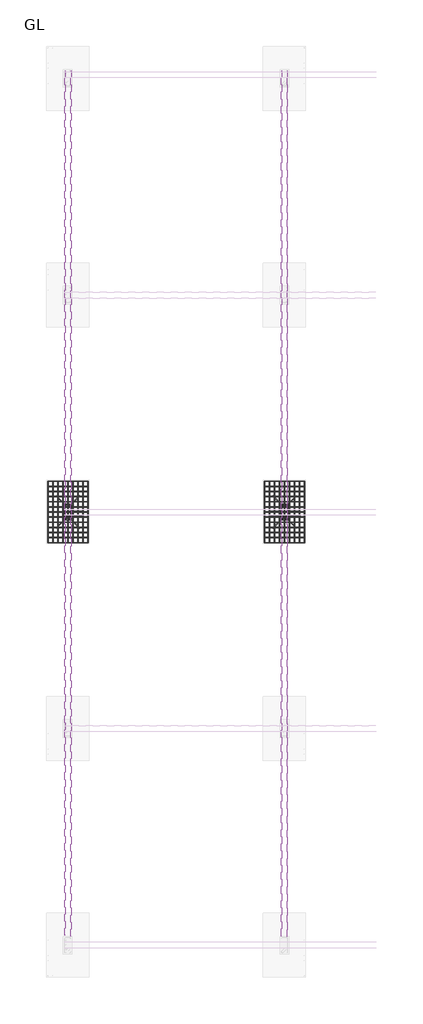
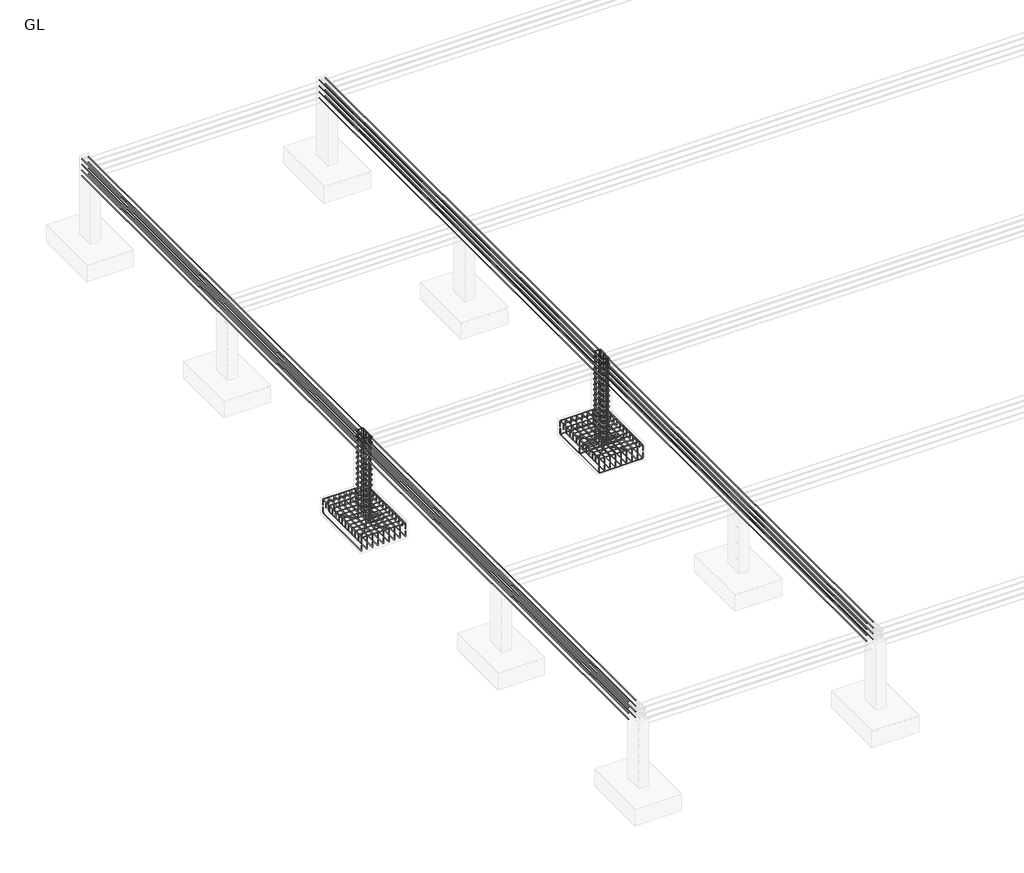
# One storey, part 5 of 16: 24 reinforcing bars.
"""IFC4 building model written with IfcOpenShell, lengths in millimetres."""

from ifc_helpers import new_model, si_unit, point, frame, origin, place, context, project, spatial, polyline, circle_curve, trimmed, segment, composite_curve, source, transform, mapped, element, save
from ifc_brep_helpers import swept_disk

model = new_model("IFC4")

# Units and contexts
model_context = context("Model", 3, world=origin())
ifc_project = project(units=[si_unit("LENGTHUNIT", "METRE", prefix="MILLI")], contexts=[model_context])

# Site, building, storey
site = spatial("IfcSite", under=ifc_project)
building = spatial("IfcBuilding", under=site)
storey = spatial("IfcBuildingStorey", under=building, Name="GL", Elevation=-1829.0)

# Reinforcing bars
placement = place(None, origin())
reinforcing_bar_shape = source(origin(), model_context, "Body", "SolidModel", [
    swept_disk(composite_curve([segment(polyline([(-23370.9544379, -7223.1167521, -2022.436678), (-23370.9544379, -7223.1167521, -1898.436678)]), True, "CONTINUOUS"), segment(trimmed(circle_curve(frame((-23340.9544379, -7223.1167521, -1898.436678), z_axis=(0.0, 1.0, 0.0), x_axis=(-30.0, 0.0, 0.0)), 30.0), [point((-23370.9544379, -7223.1167521, -1898.436678))], [point((-23340.9544379, -7223.1167521, -1868.436678))], True, "CARTESIAN"), True, "CONTINUOUS"), segment(polyline([(-23340.9544379, -7223.1167521, -1868.436678), (-22272.9544379, -7223.1167521, -1868.436678)]), True, "CONTINUOUS"), segment(trimmed(circle_curve(frame((-22272.9544379, -7223.1167521, -1898.436678), z_axis=(0.0, 1.0, 0.0), x_axis=(0.0, 0.0, 30.0)), 30.0), [point((-22272.9544379, -7223.1167521, -1868.436678))], [point((-22242.9544379, -7223.1167521, -1898.436678))], True, "CARTESIAN"), True, "CONTINUOUS"), segment(polyline([(-22242.9544379, -7223.1167521, -1898.436678), (-22242.9544379, -7223.1167521, -2022.436678)]), True, "CONTINUOUS")], self_intersect=False), 6.0),
])
element("IfcReinforcingBar", 1, at=placement, inside=storey, context=model_context, shape_type="MappedRepresentation", body=[
    mapped(reinforcing_bar_shape, transform((0.0, 0.0, 0.0), x_axis=(1.0, 0.0, 0.0), y_axis=(0.0, 1.0, 0.0), z_axis=(0.0, 0.0, 1.0))),
    mapped(reinforcing_bar_shape, transform((0.0, -144.0, 0.0), x_axis=(1.0, 0.0, 0.0), y_axis=(0.0, 1.0, 0.0), z_axis=(0.0, 0.0, 1.0))),
    mapped(reinforcing_bar_shape, transform((0.0, -288.0, 0.0), x_axis=(1.0, 0.0, 0.0), y_axis=(0.0, 1.0, 0.0), z_axis=(0.0, 0.0, 1.0))),
    mapped(reinforcing_bar_shape, transform((0.0, -432.0, 0.0), x_axis=(1.0, 0.0, 0.0), y_axis=(0.0, 1.0, 0.0), z_axis=(0.0, 0.0, 1.0))),
    mapped(reinforcing_bar_shape, transform((0.0, -576.0, 0.0), x_axis=(1.0, 0.0, 0.0), y_axis=(0.0, 1.0, 0.0), z_axis=(0.0, 0.0, 1.0))),
    mapped(reinforcing_bar_shape, transform((0.0, -720.0, 0.0), x_axis=(1.0, 0.0, 0.0), y_axis=(0.0, 1.0, 0.0), z_axis=(0.0, 0.0, 1.0))),
    mapped(reinforcing_bar_shape, transform((0.0, -864.0, 0.0), x_axis=(1.0, 0.0, 0.0), y_axis=(0.0, 1.0, 0.0), z_axis=(0.0, 0.0, 1.0))),
    mapped(reinforcing_bar_shape, transform((0.0, -1008.0, 0.0), x_axis=(1.0, 0.0, 0.0), y_axis=(0.0, 1.0, 0.0), z_axis=(0.0, 0.0, 1.0))),
    mapped(reinforcing_bar_shape, transform((0.0, -1152.0, 0.0), x_axis=(1.0, 0.0, 0.0), y_axis=(0.0, 1.0, 0.0), z_axis=(0.0, 0.0, 1.0))),
    mapped(reinforcing_bar_shape, transform((0.0, -1296.0, 0.0), x_axis=(1.0, 0.0, 0.0), y_axis=(0.0, 1.0, 0.0), z_axis=(0.0, 0.0, 1.0))),
    mapped(reinforcing_bar_shape, transform((0.0, -1440.0, 0.0), x_axis=(1.0, 0.0, 0.0), y_axis=(0.0, 1.0, 0.0), z_axis=(0.0, 0.0, 1.0))),
    mapped(reinforcing_bar_shape, transform((0.0, -1584.0, 0.0), x_axis=(1.0, 0.0, 0.0), y_axis=(0.0, 1.0, 0.0), z_axis=(0.0, 0.0, 1.0))),
    mapped(reinforcing_bar_shape, transform((0.0, -1728.0, 0.0), x_axis=(1.0, 0.0, 0.0), y_axis=(0.0, 1.0, 0.0), z_axis=(0.0, 0.0, 1.0))),
])
reinforcing_bar_2_shape = source(origin(), model_context, "Body", "SolidModel", [
    swept_disk(composite_curve([segment(polyline([(-23370.9544379, -8951.1167521, -2027.5081232), (-23370.9544379, -8951.1167521, -1903.5081232)]), True, "CONTINUOUS"), segment(trimmed(circle_curve(frame((-23370.9544379, -8921.1167521, -1903.5081232), z_axis=(-1.0, 0.0, 0.0), x_axis=(0.0, -30.0, 0.0)), 30.0), [point((-23370.9544379, -8951.1167521, -1903.5081232))], [point((-23370.9544379, -8921.1167521, -1873.5081232))], True, "CARTESIAN"), True, "CONTINUOUS"), segment(polyline([(-23370.9544379, -8921.1167521, -1873.5081232), (-23370.9544379, -7253.1167521, -1873.5081232)]), True, "CONTINUOUS"), segment(trimmed(circle_curve(frame((-23370.9544379, -7253.1167521, -1903.5081232), z_axis=(-1.0, 0.0, 0.0), x_axis=(0.0, 0.0, 30.0)), 30.0), [point((-23370.9544379, -7253.1167521, -1873.5081232))], [point((-23370.9544379, -7223.1167521, -1903.5081232))], True, "CARTESIAN"), True, "CONTINUOUS"), segment(polyline([(-23370.9544379, -7223.1167521, -1903.5081232), (-23370.9544379, -7223.1167521, -2027.5081232)]), True, "CONTINUOUS")], self_intersect=False), 6.0),
])
element("IfcReinforcingBar", 2, at=placement, inside=storey, context=model_context, shape_type="MappedRepresentation", body=[
    mapped(reinforcing_bar_2_shape, transform((0.0, 0.0, 0.0), x_axis=(1.0, 0.0, 0.0), y_axis=(0.0, 1.0, 0.0), z_axis=(0.0, 0.0, 1.0))),
    mapped(reinforcing_bar_2_shape, transform((141.0, 0.0, 0.0), x_axis=(1.0, 0.0, 0.0), y_axis=(0.0, 1.0, 0.0), z_axis=(0.0, 0.0, 1.0))),
    mapped(reinforcing_bar_2_shape, transform((282.0, 0.0, 0.0), x_axis=(1.0, 0.0, 0.0), y_axis=(0.0, 1.0, 0.0), z_axis=(0.0, 0.0, 1.0))),
    mapped(reinforcing_bar_2_shape, transform((423.0, 0.0, 0.0), x_axis=(1.0, 0.0, 0.0), y_axis=(0.0, 1.0, 0.0), z_axis=(0.0, 0.0, 1.0))),
    mapped(reinforcing_bar_2_shape, transform((564.0, 0.0, 0.0), x_axis=(1.0, 0.0, 0.0), y_axis=(0.0, 1.0, 0.0), z_axis=(0.0, 0.0, 1.0))),
    mapped(reinforcing_bar_2_shape, transform((705.0, 0.0, 0.0), x_axis=(1.0, 0.0, 0.0), y_axis=(0.0, 1.0, 0.0), z_axis=(0.0, 0.0, 1.0))),
    mapped(reinforcing_bar_2_shape, transform((846.0, 0.0, 0.0), x_axis=(1.0, 0.0, 0.0), y_axis=(0.0, 1.0, 0.0), z_axis=(0.0, 0.0, 1.0))),
    mapped(reinforcing_bar_2_shape, transform((987.0, 0.0, 0.0), x_axis=(1.0, 0.0, 0.0), y_axis=(0.0, 1.0, 0.0), z_axis=(0.0, 0.0, 1.0))),
    mapped(reinforcing_bar_2_shape, transform((1128.0, 0.0, 0.0), x_axis=(1.0, 0.0, 0.0), y_axis=(0.0, 1.0, 0.0), z_axis=(0.0, 0.0, 1.0))),
])
reinforcing_bar_3_shape = source(origin(), model_context, "Body", "SolidModel", [
    swept_disk(composite_curve([segment(polyline([(-22242.9544379, -8951.1167521, -2080.6239909), (-22242.9544379, -8951.1167521, -2204.6239909)]), True, "CONTINUOUS"), segment(trimmed(circle_curve(frame((-22242.9544379, -8921.1167521, -2204.6239909), z_axis=(1.0, 0.0, 0.0), x_axis=(0.0, -30.0, 0.0)), 30.0), [point((-22242.9544379, -8951.1167521, -2204.6239909))], [point((-22242.9544379, -8921.1167521, -2234.6239909))], True, "CARTESIAN"), True, "CONTINUOUS"), segment(polyline([(-22242.9544379, -8921.1167521, -2234.6239909), (-22242.9544379, -7266.1421892, -2234.6239909)]), True, "CONTINUOUS"), segment(trimmed(circle_curve(frame((-22242.9544379, -7266.1421892, -2204.6239909), z_axis=(1.0, 0.0, 0.0), x_axis=(0.0, 0.0, -30.0)), 30.0), [point((-22242.9544379, -7266.1421892, -2234.6239909))], [point((-22242.9544379, -7236.1421892, -2204.6239909))], True, "CARTESIAN"), True, "CONTINUOUS"), segment(polyline([(-22242.9544379, -7236.1421892, -2204.6239909), (-22242.9544379, -7236.1421892, -2080.6239909)]), True, "CONTINUOUS")], self_intersect=False), 6.0),
])
element("IfcReinforcingBar", 3, at=placement, inside=storey, context=model_context, shape_type="MappedRepresentation", body=[
    mapped(reinforcing_bar_3_shape, transform((0.0, 0.0, 0.0), x_axis=(1.0, 0.0, 0.0), y_axis=(0.0, 1.0, 0.0), z_axis=(0.0, 0.0, 1.0))),
    mapped(reinforcing_bar_3_shape, transform((-141.0, 0.0, 0.0), x_axis=(1.0, 0.0, 0.0), y_axis=(0.0, 1.0, 0.0), z_axis=(0.0, 0.0, 1.0))),
    mapped(reinforcing_bar_3_shape, transform((-282.0, 0.0, 0.0), x_axis=(1.0, 0.0, 0.0), y_axis=(0.0, 1.0, 0.0), z_axis=(0.0, 0.0, 1.0))),
    mapped(reinforcing_bar_3_shape, transform((-423.0, 0.0, 0.0), x_axis=(1.0, 0.0, 0.0), y_axis=(0.0, 1.0, 0.0), z_axis=(0.0, 0.0, 1.0))),
    mapped(reinforcing_bar_3_shape, transform((-564.0, 0.0, 0.0), x_axis=(1.0, 0.0, 0.0), y_axis=(0.0, 1.0, 0.0), z_axis=(0.0, 0.0, 1.0))),
    mapped(reinforcing_bar_3_shape, transform((-705.0, 0.0, 0.0), x_axis=(1.0, 0.0, 0.0), y_axis=(0.0, 1.0, 0.0), z_axis=(0.0, 0.0, 1.0))),
    mapped(reinforcing_bar_3_shape, transform((-846.0, 0.0, 0.0), x_axis=(1.0, 0.0, 0.0), y_axis=(0.0, 1.0, 0.0), z_axis=(0.0, 0.0, 1.0))),
    mapped(reinforcing_bar_3_shape, transform((-987.0, 0.0, 0.0), x_axis=(1.0, 0.0, 0.0), y_axis=(0.0, 1.0, 0.0), z_axis=(0.0, 0.0, 1.0))),
    mapped(reinforcing_bar_3_shape, transform((-1128.0, 0.0, 0.0), x_axis=(1.0, 0.0, 0.0), y_axis=(0.0, 1.0, 0.0), z_axis=(0.0, 0.0, 1.0))),
])
reinforcing_bar_4_shape = source(origin(), model_context, "Body", "SolidModel", [
    swept_disk(composite_curve([segment(polyline([(-16146.9544379, -7223.1167521, -2089.0), (-16146.9544379, -7223.1167521, -2213.0)]), True, "CONTINUOUS"), segment(trimmed(circle_curve(frame((-16176.9544379, -7223.1167521, -2213.0), z_axis=(0.0, 1.0, 0.0), x_axis=(30.0, 0.0, 0.0)), 30.0), [point((-16146.9544379, -7223.1167521, -2213.0))], [point((-16176.9544379, -7223.1167521, -2243.0))], True, "CARTESIAN"), True, "CONTINUOUS"), segment(polyline([(-16176.9544379, -7223.1167521, -2243.0), (-17244.9544379, -7223.1167521, -2243.0)]), True, "CONTINUOUS"), segment(trimmed(circle_curve(frame((-17244.9544379, -7223.1167521, -2213.0), z_axis=(0.0, 1.0, 0.0), x_axis=(0.0, 0.0, -30.0)), 30.0), [point((-17244.9544379, -7223.1167521, -2243.0))], [point((-17274.9544379, -7223.1167521, -2213.0))], True, "CARTESIAN"), True, "CONTINUOUS"), segment(polyline([(-17274.9544379, -7223.1167521, -2213.0), (-17274.9544379, -7223.1167521, -2089.0)]), True, "CONTINUOUS")], self_intersect=False), 6.0),
])
element("IfcReinforcingBar", 4, at=placement, inside=storey, context=model_context, shape_type="MappedRepresentation", body=[
    mapped(reinforcing_bar_4_shape, transform((0.0, 0.0, 0.0), x_axis=(1.0, 0.0, 0.0), y_axis=(0.0, 1.0, 0.0), z_axis=(0.0, 0.0, 1.0))),
    mapped(reinforcing_bar_4_shape, transform((0.0, -864.0, 0.0), x_axis=(1.0, 0.0, 0.0), y_axis=(0.0, 1.0, 0.0), z_axis=(0.0, 0.0, 1.0))),
    mapped(reinforcing_bar_4_shape, transform((0.0, -1728.0, 0.0), x_axis=(1.0, 0.0, 0.0), y_axis=(0.0, 1.0, 0.0), z_axis=(0.0, 0.0, 1.0))),
])
reinforcing_bar_5_shape = source(origin(), model_context, "Body", "SolidModel", [
    swept_disk(composite_curve([segment(polyline([(-17274.9544379, -7223.1167521, -2022.436678), (-17274.9544379, -7223.1167521, -1898.436678)]), True, "CONTINUOUS"), segment(trimmed(circle_curve(frame((-17244.9544379, -7223.1167521, -1898.436678), z_axis=(0.0, 1.0, 0.0), x_axis=(-30.0, 0.0, 0.0)), 30.0), [point((-17274.9544379, -7223.1167521, -1898.436678))], [point((-17244.9544379, -7223.1167521, -1868.436678))], True, "CARTESIAN"), True, "CONTINUOUS"), segment(polyline([(-17244.9544379, -7223.1167521, -1868.436678), (-16176.9544379, -7223.1167521, -1868.436678)]), True, "CONTINUOUS"), segment(trimmed(circle_curve(frame((-16176.9544379, -7223.1167521, -1898.436678), z_axis=(0.0, 1.0, 0.0), x_axis=(0.0, 0.0, 30.0)), 30.0), [point((-16176.9544379, -7223.1167521, -1868.436678))], [point((-16146.9544379, -7223.1167521, -1898.436678))], True, "CARTESIAN"), True, "CONTINUOUS"), segment(polyline([(-16146.9544379, -7223.1167521, -1898.436678), (-16146.9544379, -7223.1167521, -2022.436678)]), True, "CONTINUOUS")], self_intersect=False), 6.0),
])
element("IfcReinforcingBar", 5, at=placement, inside=storey, context=model_context, shape_type="MappedRepresentation", body=[
    mapped(reinforcing_bar_5_shape, transform((0.0, 0.0, 0.0), x_axis=(1.0, 0.0, 0.0), y_axis=(0.0, 1.0, 0.0), z_axis=(0.0, 0.0, 1.0))),
    mapped(reinforcing_bar_5_shape, transform((0.0, -144.0, 0.0), x_axis=(1.0, 0.0, 0.0), y_axis=(0.0, 1.0, 0.0), z_axis=(0.0, 0.0, 1.0))),
    mapped(reinforcing_bar_5_shape, transform((0.0, -288.0, 0.0), x_axis=(1.0, 0.0, 0.0), y_axis=(0.0, 1.0, 0.0), z_axis=(0.0, 0.0, 1.0))),
    mapped(reinforcing_bar_5_shape, transform((0.0, -432.0, 0.0), x_axis=(1.0, 0.0, 0.0), y_axis=(0.0, 1.0, 0.0), z_axis=(0.0, 0.0, 1.0))),
    mapped(reinforcing_bar_5_shape, transform((0.0, -576.0, 0.0), x_axis=(1.0, 0.0, 0.0), y_axis=(0.0, 1.0, 0.0), z_axis=(0.0, 0.0, 1.0))),
    mapped(reinforcing_bar_5_shape, transform((0.0, -720.0, 0.0), x_axis=(1.0, 0.0, 0.0), y_axis=(0.0, 1.0, 0.0), z_axis=(0.0, 0.0, 1.0))),
    mapped(reinforcing_bar_5_shape, transform((0.0, -864.0, 0.0), x_axis=(1.0, 0.0, 0.0), y_axis=(0.0, 1.0, 0.0), z_axis=(0.0, 0.0, 1.0))),
    mapped(reinforcing_bar_5_shape, transform((0.0, -1008.0, 0.0), x_axis=(1.0, 0.0, 0.0), y_axis=(0.0, 1.0, 0.0), z_axis=(0.0, 0.0, 1.0))),
    mapped(reinforcing_bar_5_shape, transform((0.0, -1152.0, 0.0), x_axis=(1.0, 0.0, 0.0), y_axis=(0.0, 1.0, 0.0), z_axis=(0.0, 0.0, 1.0))),
    mapped(reinforcing_bar_5_shape, transform((0.0, -1296.0, 0.0), x_axis=(1.0, 0.0, 0.0), y_axis=(0.0, 1.0, 0.0), z_axis=(0.0, 0.0, 1.0))),
    mapped(reinforcing_bar_5_shape, transform((0.0, -1440.0, 0.0), x_axis=(1.0, 0.0, 0.0), y_axis=(0.0, 1.0, 0.0), z_axis=(0.0, 0.0, 1.0))),
    mapped(reinforcing_bar_5_shape, transform((0.0, -1584.0, 0.0), x_axis=(1.0, 0.0, 0.0), y_axis=(0.0, 1.0, 0.0), z_axis=(0.0, 0.0, 1.0))),
    mapped(reinforcing_bar_5_shape, transform((0.0, -1728.0, 0.0), x_axis=(1.0, 0.0, 0.0), y_axis=(0.0, 1.0, 0.0), z_axis=(0.0, 0.0, 1.0))),
])
reinforcing_bar_6_shape = source(origin(), model_context, "Body", "SolidModel", [
    swept_disk(composite_curve([segment(polyline([(-17274.9544379, -8951.1167521, -2027.5081232), (-17274.9544379, -8951.1167521, -1903.5081232)]), True, "CONTINUOUS"), segment(trimmed(circle_curve(frame((-17274.9544379, -8921.1167521, -1903.5081232), z_axis=(-1.0, 0.0, 0.0), x_axis=(0.0, -30.0, 0.0)), 30.0), [point((-17274.9544379, -8951.1167521, -1903.5081232))], [point((-17274.9544379, -8921.1167521, -1873.5081232))], True, "CARTESIAN"), True, "CONTINUOUS"), segment(polyline([(-17274.9544379, -8921.1167521, -1873.5081232), (-17274.9544379, -7253.1167521, -1873.5081232)]), True, "CONTINUOUS"), segment(trimmed(circle_curve(frame((-17274.9544379, -7253.1167521, -1903.5081232), z_axis=(-1.0, 0.0, 0.0), x_axis=(0.0, 0.0, 30.0)), 30.0), [point((-17274.9544379, -7253.1167521, -1873.5081232))], [point((-17274.9544379, -7223.1167521, -1903.5081232))], True, "CARTESIAN"), True, "CONTINUOUS"), segment(polyline([(-17274.9544379, -7223.1167521, -1903.5081232), (-17274.9544379, -7223.1167521, -2027.5081232)]), True, "CONTINUOUS")], self_intersect=False), 6.0),
])
element("IfcReinforcingBar", 6, at=placement, inside=storey, context=model_context, shape_type="MappedRepresentation", body=[
    mapped(reinforcing_bar_6_shape, transform((0.0, 0.0, 0.0), x_axis=(1.0, 0.0, 0.0), y_axis=(0.0, 1.0, 0.0), z_axis=(0.0, 0.0, 1.0))),
    mapped(reinforcing_bar_6_shape, transform((141.0, 0.0, 0.0), x_axis=(1.0, 0.0, 0.0), y_axis=(0.0, 1.0, 0.0), z_axis=(0.0, 0.0, 1.0))),
    mapped(reinforcing_bar_6_shape, transform((282.0, 0.0, 0.0), x_axis=(1.0, 0.0, 0.0), y_axis=(0.0, 1.0, 0.0), z_axis=(0.0, 0.0, 1.0))),
    mapped(reinforcing_bar_6_shape, transform((423.0, 0.0, 0.0), x_axis=(1.0, 0.0, 0.0), y_axis=(0.0, 1.0, 0.0), z_axis=(0.0, 0.0, 1.0))),
    mapped(reinforcing_bar_6_shape, transform((564.0, 0.0, 0.0), x_axis=(1.0, 0.0, 0.0), y_axis=(0.0, 1.0, 0.0), z_axis=(0.0, 0.0, 1.0))),
    mapped(reinforcing_bar_6_shape, transform((705.0, 0.0, 0.0), x_axis=(1.0, 0.0, 0.0), y_axis=(0.0, 1.0, 0.0), z_axis=(0.0, 0.0, 1.0))),
    mapped(reinforcing_bar_6_shape, transform((846.0, 0.0, 0.0), x_axis=(1.0, 0.0, 0.0), y_axis=(0.0, 1.0, 0.0), z_axis=(0.0, 0.0, 1.0))),
    mapped(reinforcing_bar_6_shape, transform((987.0, 0.0, 0.0), x_axis=(1.0, 0.0, 0.0), y_axis=(0.0, 1.0, 0.0), z_axis=(0.0, 0.0, 1.0))),
    mapped(reinforcing_bar_6_shape, transform((1128.0, 0.0, 0.0), x_axis=(1.0, 0.0, 0.0), y_axis=(0.0, 1.0, 0.0), z_axis=(0.0, 0.0, 1.0))),
])
reinforcing_bar_7_shape = source(origin(), model_context, "Body", "SolidModel", [
    swept_disk(composite_curve([segment(polyline([(-16146.9544379, -8951.1167521, -2080.6239909), (-16146.9544379, -8951.1167521, -2204.6239909)]), True, "CONTINUOUS"), segment(trimmed(circle_curve(frame((-16146.9544379, -8921.1167521, -2204.6239909), z_axis=(1.0, 0.0, 0.0), x_axis=(0.0, -30.0, 0.0)), 30.0), [point((-16146.9544379, -8951.1167521, -2204.6239909))], [point((-16146.9544379, -8921.1167521, -2234.6239909))], True, "CARTESIAN"), True, "CONTINUOUS"), segment(polyline([(-16146.9544379, -8921.1167521, -2234.6239909), (-16146.9544379, -7266.1421892, -2234.6239909)]), True, "CONTINUOUS"), segment(trimmed(circle_curve(frame((-16146.9544379, -7266.1421892, -2204.6239909), z_axis=(1.0, 0.0, 0.0), x_axis=(0.0, 0.0, -30.0)), 30.0), [point((-16146.9544379, -7266.1421892, -2234.6239909))], [point((-16146.9544379, -7236.1421892, -2204.6239909))], True, "CARTESIAN"), True, "CONTINUOUS"), segment(polyline([(-16146.9544379, -7236.1421892, -2204.6239909), (-16146.9544379, -7236.1421892, -2080.6239909)]), True, "CONTINUOUS")], self_intersect=False), 6.0),
])
element("IfcReinforcingBar", 7, at=placement, inside=storey, context=model_context, shape_type="MappedRepresentation", body=[
    mapped(reinforcing_bar_7_shape, transform((0.0, 0.0, 0.0), x_axis=(1.0, 0.0, 0.0), y_axis=(0.0, 1.0, 0.0), z_axis=(0.0, 0.0, 1.0))),
    mapped(reinforcing_bar_7_shape, transform((-141.0, 0.0, 0.0), x_axis=(1.0, 0.0, 0.0), y_axis=(0.0, 1.0, 0.0), z_axis=(0.0, 0.0, 1.0))),
    mapped(reinforcing_bar_7_shape, transform((-282.0, 0.0, 0.0), x_axis=(1.0, 0.0, 0.0), y_axis=(0.0, 1.0, 0.0), z_axis=(0.0, 0.0, 1.0))),
    mapped(reinforcing_bar_7_shape, transform((-423.0, 0.0, 0.0), x_axis=(1.0, 0.0, 0.0), y_axis=(0.0, 1.0, 0.0), z_axis=(0.0, 0.0, 1.0))),
    mapped(reinforcing_bar_7_shape, transform((-564.0, 0.0, 0.0), x_axis=(1.0, 0.0, 0.0), y_axis=(0.0, 1.0, 0.0), z_axis=(0.0, 0.0, 1.0))),
    mapped(reinforcing_bar_7_shape, transform((-705.0, 0.0, 0.0), x_axis=(1.0, 0.0, 0.0), y_axis=(0.0, 1.0, 0.0), z_axis=(0.0, 0.0, 1.0))),
    mapped(reinforcing_bar_7_shape, transform((-846.0, 0.0, 0.0), x_axis=(1.0, 0.0, 0.0), y_axis=(0.0, 1.0, 0.0), z_axis=(0.0, 0.0, 1.0))),
    mapped(reinforcing_bar_7_shape, transform((-987.0, 0.0, 0.0), x_axis=(1.0, 0.0, 0.0), y_axis=(0.0, 1.0, 0.0), z_axis=(0.0, 0.0, 1.0))),
    mapped(reinforcing_bar_7_shape, transform((-1128.0, 0.0, 0.0), x_axis=(1.0, 0.0, 0.0), y_axis=(0.0, 1.0, 0.0), z_axis=(0.0, 0.0, 1.0))),
])
reinforcing_bar_8_shape = source(origin(), model_context, "Body", "SolidModel", [
    swept_disk(composite_curve([segment(polyline([(-16703.4864005, -8162.2223078, -1793.0), (-16791.1676414, -8249.9035486, -1793.0)]), True, "CONTINUOUS"), segment(trimmed(circle_curve(frame((-16769.9544379, -8271.1167521, -1793.0), z_axis=(0.0, 0.0, 1.0), x_axis=(-21.21320349999951, 21.213203500001327, 0.0)), 30.0), [point((-16791.1676414, -8249.9035486, -1793.0))], [point((-16769.9544379, -8301.1167521, -1793.0))], True, "CARTESIAN"), True, "CONTINUOUS"), segment(polyline([(-16769.9544379, -8301.1167521, -1793.0), (-16651.9544379, -8301.1167521, -1793.0)]), True, "CONTINUOUS"), segment(trimmed(circle_curve(frame((-16651.9544379, -8271.1167521, -1793.0), z_axis=(0.0, 0.0, 1.0), x_axis=(0.0, -30.0, 0.0)), 30.0), [point((-16651.9544379, -8301.1167521, -1793.0))], [point((-16621.9544379, -8271.1167521, -1793.0))], True, "CARTESIAN"), True, "CONTINUOUS"), segment(polyline([(-16621.9544379, -8271.1167521, -1793.0), (-16621.9544379, -7903.1167521, -1793.0)]), True, "CONTINUOUS"), segment(trimmed(circle_curve(frame((-16651.8864962, -7903.1167521, -1795.0178916), z_axis=(-0.06726305234213417, 0.0, 0.9977352764083365), x_axis=(29.93205830000079, 0.0, 2.0178915999999845)), 30.0), [point((-16621.9544379, -7903.1167521, -1793.0))], [point((-16651.8864962, -7873.1167521, -1795.0178916))], True, "CARTESIAN"), True, "CONTINUOUS"), segment(polyline([(-16651.8864962, -7873.1167521, -1795.0178916), (-16770.0223796, -7873.1167521, -1802.9821084)]), True, "CONTINUOUS"), segment(trimmed(circle_curve(frame((-16770.0223796, -7903.1167521, -1802.9821084), z_axis=(-0.06726305234213417, 0.0, 0.9977352764083365), x_axis=(0.0, 30.0, 0.0)), 30.0), [point((-16770.0223796, -7873.1167521, -1802.9821084))], [point((-16799.9544379, -7903.1167521, -1805.0))], True, "CARTESIAN"), True, "CONTINUOUS"), segment(polyline([(-16799.9544379, -7903.1167521, -1805.0), (-16799.9544379, -8271.1167521, -1805.0)]), True, "CONTINUOUS"), segment(trimmed(circle_curve(frame((-16769.9544379, -8271.1167521, -1805.0), z_axis=(0.0, 0.0, 1.0), x_axis=(-30.0, 0.0, 0.0)), 30.0), [point((-16799.9544379, -8271.1167521, -1805.0))], [point((-16748.7412345, -8292.3299555, -1805.0))], True, "CARTESIAN"), True, "CONTINUOUS"), segment(polyline([(-16748.7412345, -8292.3299555, -1805.0), (-16661.0599936, -8204.6487146, -1805.0)]), True, "CONTINUOUS")], self_intersect=False), 6.0),
])
element("IfcReinforcingBar", 8, at=placement, inside=storey, context=model_context, shape_type="MappedRepresentation", body=[
    mapped(reinforcing_bar_8_shape, transform((0.0, 0.0, 0.0), x_axis=(1.0, 0.0, 0.0), y_axis=(0.0, 1.0, 0.0), z_axis=(0.0, 0.0, 1.0))),
    mapped(reinforcing_bar_8_shape, transform((0.0, 0.0, 144.8571429), x_axis=(1.0, 0.0, 0.0), y_axis=(0.0, 1.0, 0.0), z_axis=(0.0, 0.0, 1.0))),
    mapped(reinforcing_bar_8_shape, transform((0.0, 0.0, 289.7142857), x_axis=(1.0, 0.0, 0.0), y_axis=(0.0, 1.0, 0.0), z_axis=(0.0, 0.0, 1.0))),
    mapped(reinforcing_bar_8_shape, transform((0.0, 0.0, 434.5714286), x_axis=(1.0, 0.0, 0.0), y_axis=(0.0, 1.0, 0.0), z_axis=(0.0, 0.0, 1.0))),
    mapped(reinforcing_bar_8_shape, transform((0.0, 0.0, 579.4285714), x_axis=(1.0, 0.0, 0.0), y_axis=(0.0, 1.0, 0.0), z_axis=(0.0, 0.0, 1.0))),
    mapped(reinforcing_bar_8_shape, transform((0.0, 0.0, 724.2857143), x_axis=(1.0, 0.0, 0.0), y_axis=(0.0, 1.0, 0.0), z_axis=(0.0, 0.0, 1.0))),
    mapped(reinforcing_bar_8_shape, transform((0.0, 0.0, 869.1428571), x_axis=(1.0, 0.0, 0.0), y_axis=(0.0, 1.0, 0.0), z_axis=(0.0, 0.0, 1.0))),
    mapped(reinforcing_bar_8_shape, transform((0.0, 0.0, 1014.0), x_axis=(1.0, 0.0, 0.0), y_axis=(0.0, 1.0, 0.0), z_axis=(0.0, 0.0, 1.0))),
    mapped(reinforcing_bar_8_shape, transform((0.0, 0.0, 1158.8571429), x_axis=(1.0, 0.0, 0.0), y_axis=(0.0, 1.0, 0.0), z_axis=(0.0, 0.0, 1.0))),
    mapped(reinforcing_bar_8_shape, transform((0.0, 0.0, 1303.7142857), x_axis=(1.0, 0.0, 0.0), y_axis=(0.0, 1.0, 0.0), z_axis=(0.0, 0.0, 1.0))),
    mapped(reinforcing_bar_8_shape, transform((0.0, 0.0, 1448.5714286), x_axis=(1.0, 0.0, 0.0), y_axis=(0.0, 1.0, 0.0), z_axis=(0.0, 0.0, 1.0))),
    mapped(reinforcing_bar_8_shape, transform((0.0, 0.0, 1593.4285714), x_axis=(1.0, 0.0, 0.0), y_axis=(0.0, 1.0, 0.0), z_axis=(0.0, 0.0, 1.0))),
    mapped(reinforcing_bar_8_shape, transform((0.0, 0.0, 1738.2857143), x_axis=(1.0, 0.0, 0.0), y_axis=(0.0, 1.0, 0.0), z_axis=(0.0, 0.0, 1.0))),
    mapped(reinforcing_bar_8_shape, transform((0.0, 0.0, 1883.1428571), x_axis=(1.0, 0.0, 0.0), y_axis=(0.0, 1.0, 0.0), z_axis=(0.0, 0.0, 1.0))),
    mapped(reinforcing_bar_8_shape, transform((0.0, 0.0, 2028.0), x_axis=(1.0, 0.0, 0.0), y_axis=(0.0, 1.0, 0.0), z_axis=(0.0, 0.0, 1.0))),
])
element("IfcReinforcingBar", 9, at=placement, inside=storey, context=model_context, shape_type="SolidModel", body=[
    swept_disk(composite_curve([segment(polyline([(-16768.0642232, -8272.0642439, 241.0), (-16768.0642232, -8272.0642439, -2129.0)]), True, "CONTINUOUS"), segment(trimmed(circle_curve(frame((-16789.2774266, -8293.2774473, -2129.0), z_axis=(-0.7071067811865187, 0.7071067811865764, 0.0), x_axis=(21.213203400002385, 21.213203400000566, 0.0)), 30.0), [point((-16768.0642232, -8272.0642439, -2129.0))], [point((-16789.2774266, -8293.2774473, -2159.0))], True, "CARTESIAN"), True, "CONTINUOUS"), segment(polyline([(-16789.2774266, -8293.2774473, -2159.0), (-17036.7648, -8540.7648207, -2159.0)]), True, "CONTINUOUS")], self_intersect=False), 6.0),
])
element("IfcReinforcingBar", 10, at=placement, inside=storey, context=model_context, shape_type="SolidModel", body=[
    swept_disk(composite_curve([segment(polyline([(-16768.0642232, -7902.1692603, 241.0), (-16768.0642232, -7902.1692603, -2129.0)]), True, "CONTINUOUS"), segment(trimmed(circle_curve(frame((-16789.2774266, -7880.9560568, -2129.0), z_axis=(0.7071067811865218, 0.7071067811865733, 0.0), x_axis=(21.213203400002385, -21.213203500000418, 0.0)), 30.0), [point((-16768.0642232, -7902.1692603, -2129.0))], [point((-16789.2774266, -7880.9560568, -2159.0))], True, "CARTESIAN"), True, "CONTINUOUS"), segment(polyline([(-16789.2774266, -7880.9560568, -2159.0), (-17036.7648, -7633.4686834, -2159.0)]), True, "CONTINUOUS")], self_intersect=False), 6.0),
])
element("IfcReinforcingBar", 11, at=placement, inside=storey, context=model_context, shape_type="SolidModel", body=[
    swept_disk(composite_curve([segment(polyline([(-16653.8446527, -8272.0642439, 241.0), (-16653.8446527, -8272.0642439, -2129.0)]), True, "CONTINUOUS"), segment(trimmed(circle_curve(frame((-16632.6314492, -8293.2774473, -2129.0), z_axis=(-0.7071067811865248, -0.7071067811865703, 0.0), x_axis=(-21.213203500003146, 21.213203400000566, 0.0)), 30.0), [point((-16653.8446527, -8272.0642439, -2129.0))], [point((-16632.6314492, -8293.2774473, -2159.0))], True, "CARTESIAN"), True, "CONTINUOUS"), segment(polyline([(-16632.6314492, -8293.2774473, -2159.0), (-16385.1440758, -8540.7648207, -2159.0)]), True, "CONTINUOUS")], self_intersect=False), 6.0),
])
element("IfcReinforcingBar", 12, at=placement, inside=storey, context=model_context, shape_type="SolidModel", body=[
    swept_disk(composite_curve([segment(polyline([(-16653.8446527, -7902.1692603, 241.0), (-16653.8446527, -7902.1692603, -2129.0)]), True, "CONTINUOUS"), segment(trimmed(circle_curve(frame((-16632.6314492, -7880.9560568, -2129.0), z_axis=(0.7071067811865157, -0.7071067811865794, 0.0), x_axis=(-21.213203500003146, -21.213203500000418, 0.0)), 30.0), [point((-16653.8446527, -7902.1692603, -2129.0))], [point((-16632.6314492, -7880.9560568, -2159.0))], True, "CARTESIAN"), True, "CONTINUOUS"), segment(polyline([(-16632.6314492, -7880.9560568, -2159.0), (-16385.1440758, -7633.4686834, -2159.0)]), True, "CONTINUOUS")], self_intersect=False), 6.0),
])
reinforcing_bar_9_shape = source(origin(), model_context, "Body", "SolidModel", [
    swept_disk(composite_curve([segment(polyline([(-16768.0642232, -8194.9117405, 241.0), (-16768.0642232, -8194.9117405, -2129.0)]), True, "CONTINUOUS"), segment(trimmed(circle_curve(frame((-16798.0642232, -8194.9117405, -2129.0), z_axis=(0.0, 1.0, 0.0), x_axis=(30.0, 0.0, 0.0)), 30.0), [point((-16768.0642232, -8194.9117405, -2129.0))], [point((-16798.0642232, -8194.9117405, -2159.0))], True, "CARTESIAN"), True, "CONTINUOUS"), segment(polyline([(-16798.0642232, -8194.9117405, -2159.0), (-17148.0642232, -8194.9117405, -2159.0)]), True, "CONTINUOUS")], self_intersect=False), 6.0),
])
element("IfcReinforcingBar", 13, at=placement, inside=storey, context=model_context, shape_type="MappedRepresentation", body=[
    mapped(reinforcing_bar_9_shape, transform((0.0, 0.0, 0.0), x_axis=(1.0, 0.0, 0.0), y_axis=(0.0, 1.0, 0.0), z_axis=(0.0, 0.0, 1.0))),
    mapped(reinforcing_bar_9_shape, transform((0.0, 123.5823926, 0.0), x_axis=(1.0, 0.0, 0.0), y_axis=(0.0, 1.0, 0.0), z_axis=(0.0, 0.0, 1.0))),
    mapped(reinforcing_bar_9_shape, transform((0.0, 247.1647853, 0.0), x_axis=(1.0, 0.0, 0.0), y_axis=(0.0, 1.0, 0.0), z_axis=(0.0, 0.0, 1.0))),
])
reinforcing_bar_10_shape = source(origin(), model_context, "Body", "SolidModel", [
    swept_disk(composite_curve([segment(polyline([(-16653.8446527, -8194.9117405, 241.0), (-16653.8446527, -8194.9117405, -2129.0)]), True, "CONTINUOUS"), segment(trimmed(circle_curve(frame((-16623.8446527, -8194.9117405, -2129.0), z_axis=(0.0, -1.0, 0.0), x_axis=(-30.0, 0.0, 0.0)), 30.0), [point((-16653.8446527, -8194.9117405, -2129.0))], [point((-16623.8446527, -8194.9117405, -2159.0))], True, "CARTESIAN"), True, "CONTINUOUS"), segment(polyline([(-16623.8446527, -8194.9117405, -2159.0), (-16273.8446527, -8194.9117405, -2159.0)]), True, "CONTINUOUS")], self_intersect=False), 6.0),
])
element("IfcReinforcingBar", 14, at=placement, inside=storey, context=model_context, shape_type="MappedRepresentation", body=[
    mapped(reinforcing_bar_10_shape, transform((0.0, 0.0, 0.0), x_axis=(1.0, 0.0, 0.0), y_axis=(0.0, 1.0, 0.0), z_axis=(0.0, 0.0, 1.0))),
    mapped(reinforcing_bar_10_shape, transform((0.0, 123.5823926, 0.0), x_axis=(1.0, 0.0, 0.0), y_axis=(0.0, 1.0, 0.0), z_axis=(0.0, 0.0, 1.0))),
    mapped(reinforcing_bar_10_shape, transform((0.0, 247.1647853, 0.0), x_axis=(1.0, 0.0, 0.0), y_axis=(0.0, 1.0, 0.0), z_axis=(0.0, 0.0, 1.0))),
])
reinforcing_bar_11_shape = source(origin(), model_context, "Body", "SolidModel", [
    swept_disk(composite_curve([segment(polyline([(-22799.4864005, -8162.2223078, -1793.0), (-22887.1676414, -8249.9035486, -1793.0)]), True, "CONTINUOUS"), segment(trimmed(circle_curve(frame((-22865.9544379, -8271.1167521, -1793.0), z_axis=(0.0, 0.0, 1.0), x_axis=(-21.21320349999951, 21.213203500001327, 0.0)), 30.0), [point((-22887.1676414, -8249.9035486, -1793.0))], [point((-22865.9544379, -8301.1167521, -1793.0))], True, "CARTESIAN"), True, "CONTINUOUS"), segment(polyline([(-22865.9544379, -8301.1167521, -1793.0), (-22747.9544379, -8301.1167521, -1793.0)]), True, "CONTINUOUS"), segment(trimmed(circle_curve(frame((-22747.9544379, -8271.1167521, -1793.0), z_axis=(0.0, 0.0, 1.0), x_axis=(0.0, -30.0, 0.0)), 30.0), [point((-22747.9544379, -8301.1167521, -1793.0))], [point((-22717.9544379, -8271.1167521, -1793.0))], True, "CARTESIAN"), True, "CONTINUOUS"), segment(polyline([(-22717.9544379, -8271.1167521, -1793.0), (-22717.9544379, -7903.1167521, -1793.0)]), True, "CONTINUOUS"), segment(trimmed(circle_curve(frame((-22747.8864962, -7903.1167521, -1795.0178916), z_axis=(-0.06726305234213417, 0.0, 0.9977352764083365), x_axis=(29.93205830000079, 0.0, 2.0178915999999845)), 30.0), [point((-22717.9544379, -7903.1167521, -1793.0))], [point((-22747.8864962, -7873.1167521, -1795.0178916))], True, "CARTESIAN"), True, "CONTINUOUS"), segment(polyline([(-22747.8864962, -7873.1167521, -1795.0178916), (-22866.0223796, -7873.1167521, -1802.9821084)]), True, "CONTINUOUS"), segment(trimmed(circle_curve(frame((-22866.0223796, -7903.1167521, -1802.9821084), z_axis=(-0.06726305234213417, 0.0, 0.9977352764083365), x_axis=(0.0, 30.0, 0.0)), 30.0), [point((-22866.0223796, -7873.1167521, -1802.9821084))], [point((-22895.9544379, -7903.1167521, -1805.0))], True, "CARTESIAN"), True, "CONTINUOUS"), segment(polyline([(-22895.9544379, -7903.1167521, -1805.0), (-22895.9544379, -8271.1167521, -1805.0)]), True, "CONTINUOUS"), segment(trimmed(circle_curve(frame((-22865.9544379, -8271.1167521, -1805.0), z_axis=(0.0, 0.0, 1.0), x_axis=(-30.0, 0.0, 0.0)), 30.0), [point((-22895.9544379, -8271.1167521, -1805.0))], [point((-22844.7412345, -8292.3299555, -1805.0))], True, "CARTESIAN"), True, "CONTINUOUS"), segment(polyline([(-22844.7412345, -8292.3299555, -1805.0), (-22757.0599936, -8204.6487146, -1805.0)]), True, "CONTINUOUS")], self_intersect=False), 6.0),
])
element("IfcReinforcingBar", 15, at=placement, inside=storey, context=model_context, shape_type="MappedRepresentation", body=[
    mapped(reinforcing_bar_11_shape, transform((0.0, 0.0, 0.0), x_axis=(1.0, 0.0, 0.0), y_axis=(0.0, 1.0, 0.0), z_axis=(0.0, 0.0, 1.0))),
    mapped(reinforcing_bar_11_shape, transform((0.0, 0.0, 144.8571429), x_axis=(1.0, 0.0, 0.0), y_axis=(0.0, 1.0, 0.0), z_axis=(0.0, 0.0, 1.0))),
    mapped(reinforcing_bar_11_shape, transform((0.0, 0.0, 289.7142857), x_axis=(1.0, 0.0, 0.0), y_axis=(0.0, 1.0, 0.0), z_axis=(0.0, 0.0, 1.0))),
    mapped(reinforcing_bar_11_shape, transform((0.0, 0.0, 434.5714286), x_axis=(1.0, 0.0, 0.0), y_axis=(0.0, 1.0, 0.0), z_axis=(0.0, 0.0, 1.0))),
    mapped(reinforcing_bar_11_shape, transform((0.0, 0.0, 579.4285714), x_axis=(1.0, 0.0, 0.0), y_axis=(0.0, 1.0, 0.0), z_axis=(0.0, 0.0, 1.0))),
    mapped(reinforcing_bar_11_shape, transform((0.0, 0.0, 724.2857143), x_axis=(1.0, 0.0, 0.0), y_axis=(0.0, 1.0, 0.0), z_axis=(0.0, 0.0, 1.0))),
    mapped(reinforcing_bar_11_shape, transform((0.0, 0.0, 869.1428571), x_axis=(1.0, 0.0, 0.0), y_axis=(0.0, 1.0, 0.0), z_axis=(0.0, 0.0, 1.0))),
    mapped(reinforcing_bar_11_shape, transform((0.0, 0.0, 1014.0), x_axis=(1.0, 0.0, 0.0), y_axis=(0.0, 1.0, 0.0), z_axis=(0.0, 0.0, 1.0))),
    mapped(reinforcing_bar_11_shape, transform((0.0, 0.0, 1158.8571429), x_axis=(1.0, 0.0, 0.0), y_axis=(0.0, 1.0, 0.0), z_axis=(0.0, 0.0, 1.0))),
    mapped(reinforcing_bar_11_shape, transform((0.0, 0.0, 1303.7142857), x_axis=(1.0, 0.0, 0.0), y_axis=(0.0, 1.0, 0.0), z_axis=(0.0, 0.0, 1.0))),
    mapped(reinforcing_bar_11_shape, transform((0.0, 0.0, 1448.5714286), x_axis=(1.0, 0.0, 0.0), y_axis=(0.0, 1.0, 0.0), z_axis=(0.0, 0.0, 1.0))),
    mapped(reinforcing_bar_11_shape, transform((0.0, 0.0, 1593.4285714), x_axis=(1.0, 0.0, 0.0), y_axis=(0.0, 1.0, 0.0), z_axis=(0.0, 0.0, 1.0))),
    mapped(reinforcing_bar_11_shape, transform((0.0, 0.0, 1738.2857143), x_axis=(1.0, 0.0, 0.0), y_axis=(0.0, 1.0, 0.0), z_axis=(0.0, 0.0, 1.0))),
    mapped(reinforcing_bar_11_shape, transform((0.0, 0.0, 1883.1428571), x_axis=(1.0, 0.0, 0.0), y_axis=(0.0, 1.0, 0.0), z_axis=(0.0, 0.0, 1.0))),
    mapped(reinforcing_bar_11_shape, transform((0.0, 0.0, 2028.0), x_axis=(1.0, 0.0, 0.0), y_axis=(0.0, 1.0, 0.0), z_axis=(0.0, 0.0, 1.0))),
])
element("IfcReinforcingBar", 16, at=placement, inside=storey, context=model_context, shape_type="SolidModel", body=[
    swept_disk(composite_curve([segment(polyline([(-22864.0642232, -8272.0642439, 241.0), (-22864.0642232, -8272.0642439, -2129.0)]), True, "CONTINUOUS"), segment(trimmed(circle_curve(frame((-22885.2774266, -8293.2774473, -2129.0), z_axis=(-0.7071067811865187, 0.7071067811865764, 0.0), x_axis=(21.213203400002385, 21.213203400000566, 0.0)), 30.0), [point((-22864.0642232, -8272.0642439, -2129.0))], [point((-22885.2774266, -8293.2774473, -2159.0))], True, "CARTESIAN"), True, "CONTINUOUS"), segment(polyline([(-22885.2774266, -8293.2774473, -2159.0), (-23132.7648, -8540.7648207, -2159.0)]), True, "CONTINUOUS")], self_intersect=False), 6.0),
])
element("IfcReinforcingBar", 17, at=placement, inside=storey, context=model_context, shape_type="SolidModel", body=[
    swept_disk(composite_curve([segment(polyline([(-22864.0642232, -7902.1692603, 241.0), (-22864.0642232, -7902.1692603, -2129.0)]), True, "CONTINUOUS"), segment(trimmed(circle_curve(frame((-22885.2774266, -7880.9560568, -2129.0), z_axis=(0.7071067811865218, 0.7071067811865733, 0.0), x_axis=(21.213203400002385, -21.213203500000418, 0.0)), 30.0), [point((-22864.0642232, -7902.1692603, -2129.0))], [point((-22885.2774266, -7880.9560568, -2159.0))], True, "CARTESIAN"), True, "CONTINUOUS"), segment(polyline([(-22885.2774266, -7880.9560568, -2159.0), (-23132.7648, -7633.4686834, -2159.0)]), True, "CONTINUOUS")], self_intersect=False), 6.0),
])
element("IfcReinforcingBar", 18, at=placement, inside=storey, context=model_context, shape_type="SolidModel", body=[
    swept_disk(composite_curve([segment(polyline([(-22749.8446527, -8272.0642439, 241.0), (-22749.8446527, -8272.0642439, -2129.0)]), True, "CONTINUOUS"), segment(trimmed(circle_curve(frame((-22728.6314492, -8293.2774473, -2129.0), z_axis=(-0.7071067811865248, -0.7071067811865703, 0.0), x_axis=(-21.213203500003146, 21.213203400000566, 0.0)), 30.0), [point((-22749.8446527, -8272.0642439, -2129.0))], [point((-22728.6314492, -8293.2774473, -2159.0))], True, "CARTESIAN"), True, "CONTINUOUS"), segment(polyline([(-22728.6314492, -8293.2774473, -2159.0), (-22481.1440758, -8540.7648207, -2159.0)]), True, "CONTINUOUS")], self_intersect=False), 6.0),
])
element("IfcReinforcingBar", 19, at=placement, inside=storey, context=model_context, shape_type="SolidModel", body=[
    swept_disk(composite_curve([segment(polyline([(-22749.8446527, -7902.1692603, 241.0), (-22749.8446527, -7902.1692603, -2129.0)]), True, "CONTINUOUS"), segment(trimmed(circle_curve(frame((-22728.6314492, -7880.9560568, -2129.0), z_axis=(0.7071067811865157, -0.7071067811865794, 0.0), x_axis=(-21.213203500003146, -21.213203500000418, 0.0)), 30.0), [point((-22749.8446527, -7902.1692603, -2129.0))], [point((-22728.6314492, -7880.9560568, -2159.0))], True, "CARTESIAN"), True, "CONTINUOUS"), segment(polyline([(-22728.6314492, -7880.9560568, -2159.0), (-22481.1440758, -7633.4686834, -2159.0)]), True, "CONTINUOUS")], self_intersect=False), 6.0),
])
reinforcing_bar_12_shape = source(origin(), model_context, "Body", "SolidModel", [
    swept_disk(composite_curve([segment(polyline([(-22749.8446527, -8194.9117405, 241.0), (-22749.8446527, -8194.9117405, -2129.0)]), True, "CONTINUOUS"), segment(trimmed(circle_curve(frame((-22719.8446527, -8194.9117405, -2129.0), z_axis=(0.0, -1.0, 0.0), x_axis=(-30.0, 0.0, 0.0)), 30.0), [point((-22749.8446527, -8194.9117405, -2129.0))], [point((-22719.8446527, -8194.9117405, -2159.0))], True, "CARTESIAN"), True, "CONTINUOUS"), segment(polyline([(-22719.8446527, -8194.9117405, -2159.0), (-22369.8446527, -8194.9117405, -2159.0)]), True, "CONTINUOUS")], self_intersect=False), 6.0),
])
element("IfcReinforcingBar", 20, at=placement, inside=storey, context=model_context, shape_type="MappedRepresentation", body=[
    mapped(reinforcing_bar_12_shape, transform((0.0, 0.0, 0.0), x_axis=(1.0, 0.0, 0.0), y_axis=(0.0, 1.0, 0.0), z_axis=(0.0, 0.0, 1.0))),
    mapped(reinforcing_bar_12_shape, transform((0.0, 123.5823926, 0.0), x_axis=(1.0, 0.0, 0.0), y_axis=(0.0, 1.0, 0.0), z_axis=(0.0, 0.0, 1.0))),
    mapped(reinforcing_bar_12_shape, transform((0.0, 247.1647853, 0.0), x_axis=(1.0, 0.0, 0.0), y_axis=(0.0, 1.0, 0.0), z_axis=(0.0, 0.0, 1.0))),
])
reinforcing_bar_13_shape = source(origin(), model_context, "Body", "SolidModel", [
    swept_disk(composite_curve([segment(polyline([(-22890.9544379, 4324.8832479, 204.5874893), (-22890.9544379, -19998.8393353, 204.5874893)]), True, "CONTINUOUS")], self_intersect=False), 6.0),
])
element("IfcReinforcingBar", 21, at=placement, inside=storey, context=model_context, shape_type="MappedRepresentation", body=[
    mapped(reinforcing_bar_13_shape, transform((0.0, 0.0, 0.0), x_axis=(1.0, 0.0, 0.0), y_axis=(0.0, 1.0, 0.0), z_axis=(0.0, 0.0, 1.0))),
    mapped(reinforcing_bar_13_shape, transform((0.0, 0.0, -155.681351), x_axis=(1.0, 0.0, 0.0), y_axis=(0.0, 1.0, 0.0), z_axis=(0.0, 0.0, 1.0))),
    mapped(reinforcing_bar_13_shape, transform((0.0, 0.0, -311.362702), x_axis=(1.0, 0.0, 0.0), y_axis=(0.0, 1.0, 0.0), z_axis=(0.0, 0.0, 1.0))),
    mapped(reinforcing_bar_13_shape, transform((0.0, 0.0, -467.044053), x_axis=(1.0, 0.0, 0.0), y_axis=(0.0, 1.0, 0.0), z_axis=(0.0, 0.0, 1.0))),
])
reinforcing_bar_14_shape = source(origin(), model_context, "Body", "SolidModel", [
    swept_disk(composite_curve([segment(polyline([(-22722.9544379, 4324.8832479, -262.4565636), (-22722.9544379, -20022.596908, -262.4565636)]), True, "CONTINUOUS")], self_intersect=False), 6.0),
])
element("IfcReinforcingBar", 22, at=placement, inside=storey, context=model_context, shape_type="MappedRepresentation", body=[
    mapped(reinforcing_bar_14_shape, transform((0.0, 0.0, 0.0), x_axis=(1.0, 0.0, 0.0), y_axis=(0.0, 1.0, 0.0), z_axis=(0.0, 0.0, 1.0))),
    mapped(reinforcing_bar_14_shape, transform((0.0, 0.0, 155.681351), x_axis=(1.0, 0.0, 0.0), y_axis=(0.0, 1.0, 0.0), z_axis=(0.0, 0.0, 1.0))),
    mapped(reinforcing_bar_14_shape, transform((0.0, 0.0, 311.362702), x_axis=(1.0, 0.0, 0.0), y_axis=(0.0, 1.0, 0.0), z_axis=(0.0, 0.0, 1.0))),
    mapped(reinforcing_bar_14_shape, transform((0.0, 0.0, 467.044053), x_axis=(1.0, 0.0, 0.0), y_axis=(0.0, 1.0, 0.0), z_axis=(0.0, 0.0, 1.0))),
])
reinforcing_bar_15_shape = source(origin(), model_context, "Body", "SolidModel", [
    swept_disk(composite_curve([segment(polyline([(-16794.9544379, 4324.8832479, 211.7819865), (-16794.9544379, -20015.3934205, 211.7819865)]), True, "CONTINUOUS")], self_intersect=False), 6.0),
])
element("IfcReinforcingBar", 23, at=placement, inside=storey, context=model_context, shape_type="MappedRepresentation", body=[
    mapped(reinforcing_bar_15_shape, transform((0.0, 0.0, 0.0), x_axis=(1.0, 0.0, 0.0), y_axis=(0.0, 1.0, 0.0), z_axis=(0.0, 0.0, 1.0))),
    mapped(reinforcing_bar_15_shape, transform((0.0, 0.0, -160.3962653), x_axis=(1.0, 0.0, 0.0), y_axis=(0.0, 1.0, 0.0), z_axis=(0.0, 0.0, 1.0))),
    mapped(reinforcing_bar_15_shape, transform((0.0, 0.0, -320.7925305), x_axis=(1.0, 0.0, 0.0), y_axis=(0.0, 1.0, 0.0), z_axis=(0.0, 0.0, 1.0))),
    mapped(reinforcing_bar_15_shape, transform((0.0, 0.0, -481.1887958), x_axis=(1.0, 0.0, 0.0), y_axis=(0.0, 1.0, 0.0), z_axis=(0.0, 0.0, 1.0))),
])
reinforcing_bar_16_shape = source(origin(), model_context, "Body", "SolidModel", [
    swept_disk(composite_curve([segment(polyline([(-16637.3651542, 4324.8832479, -269.4068093), (-16637.3651542, -20032.4972131, -269.4068093)]), True, "CONTINUOUS")], self_intersect=False), 6.0),
])
element("IfcReinforcingBar", 24, at=placement, inside=storey, context=model_context, shape_type="MappedRepresentation", body=[
    mapped(reinforcing_bar_16_shape, transform((0.0, 0.0, 0.0), x_axis=(1.0, 0.0, 0.0), y_axis=(0.0, 1.0, 0.0), z_axis=(0.0, 0.0, 1.0))),
    mapped(reinforcing_bar_16_shape, transform((0.0, 0.0, 160.3962653), x_axis=(1.0, 0.0, 0.0), y_axis=(0.0, 1.0, 0.0), z_axis=(0.0, 0.0, 1.0))),
    mapped(reinforcing_bar_16_shape, transform((0.0, 0.0, 320.7925305), x_axis=(1.0, 0.0, 0.0), y_axis=(0.0, 1.0, 0.0), z_axis=(0.0, 0.0, 1.0))),
    mapped(reinforcing_bar_16_shape, transform((0.0, 0.0, 481.1887958), x_axis=(1.0, 0.0, 0.0), y_axis=(0.0, 1.0, 0.0), z_axis=(0.0, 0.0, 1.0))),
])

save(model, "model.ifc")

# Revit data of these elements
# Elements 1, 2, 3, 4, 5, 6, 7, 8, 9, 10, 11, 12, 13, 14, 15, 16, 17, 18, 19, 20, 21, 22, 23, 24 (IfcReinforcingBar)
#   Phase Created = New Construction
